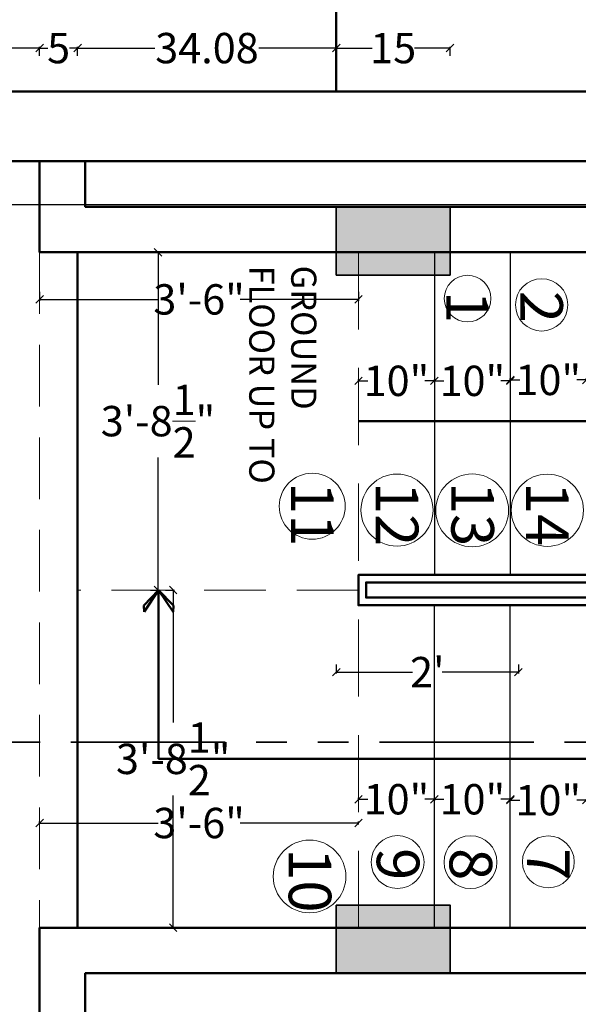
# Model space of a CAD drawing. Units: inches. Extents: x -60 to 284, y -245 to 257.
# Tile 7 of 10: x 25 to 99, y 12 to 141. Entities that reach past the tile are written whole.
import ezdxf

# ---------------------------------------------------------------- set-up
doc = ezdxf.new("R2010")
doc.units = ezdxf.units.IN
doc.header["$LTSCALE"] = 0.8
doc.header["$MEASUREMENT"] = 0
doc.linetypes.add('DASHED', pattern=[19.05, 12.7, -6.35])
doc.linetypes.add('PHANTOM', pattern=[63.5, 31.75, -6.35, 6.35, -6.35, 6.35, -6.35])
for name, color, linetype, lineweight in [('A-ANNO-DIMS', 2, 'Continuous', 18), ('A-ANNO-SECT', 1, 'PHANTOM', 35), ('A-ANNO-SYMB', 3, 'Continuous', 18), ('A-ANNO-TEXT', 3, 'Continuous', 18), ('A-ANNO-TTLB', 7, 'Continuous', 50), ('A-COLS', 1, 'Continuous', 35), ('A-FLOR-STRS', 4, 'Continuous', 25), ('A-FLOR-STRS-OVHD', 4, 'DASHED', 18), ('A-WALL', 7, 'Continuous', 50)]:
    doc.layers.add(name, color=color, linetype=linetype, lineweight=lineweight)
doc.styles.get("Standard").update_dxf_attribs({"font": 'arial.ttf'})
doc.dimstyles.get("Standard").update_dxf_attribs({"dimtxt": 4, "dimasz": 1, "dimexe": 0.18, "dimexo": 0.0625, "dimgap": 0.09, "dimtad": 0, "dimtih": 1, "dimtoh": 1, "dimzin": 0, "dimdsep": 46, "dimlunit": 4, "dimtxsty": 'Standard', "dimblk": 'OBLIQUE', "dimcen": 0.09, "dimadec": 0, "dimazin": 0, "dimtfac": 1, "dimtofl": 0, "dimtmove": 0, "dimatfit": 3, "dimfxl": 1, "dimfxlon": 1, "dimtolj": 1, "dimtzin": 0, "dimarcsym": 0})

# ---------------------------------------------------------------- blocks, each defined once
blk = doc.blocks.new('_Oblique')
at = {"color": 0, "linetype": 'ByBlock', "lineweight": -2}
blk.add_line((-0.5, -0.5), (0.5, 0.5), dxfattribs=at)
blk = doc.blocks.new('*D8')
at = {"layer": 'A-ANNO-DIMS', "color": 0, "lineweight": -2, "ltscale": 0.8, "transparency": 16777216}
for p, q in [((89.94, 38.48), (89.94, 38.66)), ((89.94, 38.48), (91.18, 38.48)), ((99.94, 38.48), (98.69, 38.48)), ((99.94, 38.6), (99.94, 38.3))]:
    blk.add_line(p, q, dxfattribs=at)
at = {"layer": 'Defpoints', "color": 0, "ltscale": 0.8, "transparency": 16777216}
for p in [(89.94, 38.48), (99.94, 38.66), (99.94, 38.48)]:
    blk.add_point(p, dxfattribs=at)
at = {"layer": 'A-ANNO-DIMS', "color": 0, "lineweight": -2, "ltscale": 0.8, "transparency": 16777216, "rotation": 180}
blk.add_blockref('_Oblique', (89.94, 38.48), dxfattribs=at)
at = {"layer": 'A-ANNO-DIMS', "color": 0, "lineweight": -2, "ltscale": 0.8, "transparency": 16777216}
blk.add_blockref('_Oblique', (99.94, 38.48), dxfattribs=at)
at = {"layer": 'A-ANNO-DIMS', "color": 0, "ltscale": 0.8, "transparency": 16777216, "insert": (94.94, 38.48), "char_height": 4, "attachment_point": 5}
blk.add_mtext('\\A1;10"', dxfattribs=at)
blk = doc.blocks.new('*D9')
at = {"layer": 'A-ANNO-DIMS', "color": 0, "lineweight": -2, "ltscale": 0.8, "transparency": 16777216}
for p, q in [((79.94, 38.54), (79.94, 38.78)), ((79.94, 38.6), (81.18, 38.6)), ((89.94, 38.6), (88.69, 38.6)), ((89.94, 38.6), (89.94, 38.78))]:
    blk.add_line(p, q, dxfattribs=at)
at = {"layer": 'Defpoints', "color": 0, "ltscale": 0.8, "transparency": 16777216}
for p in [(79.94, 38.48), (89.94, 38.6), (89.94, 38.6)]:
    blk.add_point(p, dxfattribs=at)
at = {"layer": 'A-ANNO-DIMS', "color": 0, "lineweight": -2, "ltscale": 0.8, "transparency": 16777216, "rotation": 180}
blk.add_blockref('_Oblique', (79.94, 38.6), dxfattribs=at)
at = {"layer": 'A-ANNO-DIMS', "color": 0, "lineweight": -2, "ltscale": 0.8, "transparency": 16777216}
blk.add_blockref('_Oblique', (89.94, 38.6), dxfattribs=at)
at = {"layer": 'A-ANNO-DIMS', "color": 0, "ltscale": 0.8, "transparency": 16777216, "insert": (84.94, 38.6), "char_height": 4, "attachment_point": 5}
blk.add_mtext('\\A1;10"', dxfattribs=at)
blk = doc.blocks.new('*D10')
at = {"layer": 'A-ANNO-DIMS', "color": 0, "lineweight": -2, "ltscale": 0.8, "transparency": 16777216}
for p, q in [((69.94, 38.6), (69.94, 38.78)), ((69.94, 38.6), (71.18, 38.6)), ((79.94, 38.6), (78.69, 38.6)), ((79.94, 38.72), (79.94, 38.42))]:
    blk.add_line(p, q, dxfattribs=at)
at = {"layer": 'Defpoints', "color": 0, "ltscale": 0.8, "transparency": 16777216}
for p in [(69.94, 38.6), (79.94, 38.78), (79.94, 38.6)]:
    blk.add_point(p, dxfattribs=at)
at = {"layer": 'A-ANNO-DIMS', "color": 0, "lineweight": -2, "ltscale": 0.8, "transparency": 16777216, "rotation": 180}
blk.add_blockref('_Oblique', (69.94, 38.6), dxfattribs=at)
at = {"layer": 'A-ANNO-DIMS', "color": 0, "lineweight": -2, "ltscale": 0.8, "transparency": 16777216}
blk.add_blockref('_Oblique', (79.94, 38.6), dxfattribs=at)
at = {"layer": 'A-ANNO-DIMS', "color": 0, "ltscale": 0.8, "transparency": 16777216, "insert": (74.94, 38.6), "char_height": 4, "attachment_point": 5}
blk.add_mtext('\\A1;10"', dxfattribs=at)
blk = doc.blocks.new('*D18')
at = {"layer": 'A-ANNO-DIMS', "color": 0, "lineweight": -2, "ltscale": 0.8, "transparency": 16777216}
for p, q in [((89.94, 93.85), (89.94, 94.03)), ((89.94, 93.85), (91.18, 93.85)), ((99.94, 93.85), (98.69, 93.85)), ((99.94, 93.73), (99.94, 94.03))]:
    blk.add_line(p, q, dxfattribs=at)
at = {"layer": 'Defpoints', "color": 0, "ltscale": 0.8, "transparency": 16777216}
for p in [(89.94, 93.85), (99.94, 93.85), (99.94, 93.67)]:
    blk.add_point(p, dxfattribs=at)
at = {"layer": 'A-ANNO-DIMS', "color": 0, "lineweight": -2, "ltscale": 0.8, "transparency": 16777216, "rotation": 180}
blk.add_blockref('_Oblique', (89.94, 93.85), dxfattribs=at)
at = {"layer": 'A-ANNO-DIMS', "color": 0, "lineweight": -2, "ltscale": 0.8, "transparency": 16777216}
blk.add_blockref('_Oblique', (99.94, 93.85), dxfattribs=at)
at = {"layer": 'A-ANNO-DIMS', "color": 0, "ltscale": 0.8, "transparency": 16777216, "insert": (94.94, 93.85), "char_height": 4, "attachment_point": 5}
blk.add_mtext('\\A1;10"', dxfattribs=at)
blk = doc.blocks.new('*D19')
at = {"layer": 'A-ANNO-DIMS', "color": 0, "lineweight": -2, "ltscale": 0.8, "transparency": 16777216}
for p, q in [((79.94, 93.79), (79.94, 93.55)), ((79.94, 93.73), (81.18, 93.73)), ((89.94, 93.73), (88.69, 93.73)), ((89.94, 93.73), (89.94, 93.91))]:
    blk.add_line(p, q, dxfattribs=at)
at = {"layer": 'Defpoints', "color": 0, "ltscale": 0.8, "transparency": 16777216}
for p in [(79.94, 93.85), (89.94, 93.73), (89.94, 93.73)]:
    blk.add_point(p, dxfattribs=at)
at = {"layer": 'A-ANNO-DIMS', "color": 0, "lineweight": -2, "ltscale": 0.8, "transparency": 16777216, "rotation": 180}
blk.add_blockref('_Oblique', (79.94, 93.73), dxfattribs=at)
at = {"layer": 'A-ANNO-DIMS', "color": 0, "lineweight": -2, "ltscale": 0.8, "transparency": 16777216}
blk.add_blockref('_Oblique', (89.94, 93.73), dxfattribs=at)
at = {"layer": 'A-ANNO-DIMS', "color": 0, "ltscale": 0.8, "transparency": 16777216, "insert": (84.94, 93.73), "char_height": 4, "attachment_point": 5}
blk.add_mtext('\\A1;10"', dxfattribs=at)
blk = doc.blocks.new('*D11')
at = {"layer": 'A-ANNO-DIMS', "color": 0, "lineweight": -2, "ltscale": 0.8, "transparency": 16777216}
for p, q in [((69.94, 93.73), (69.94, 93.91)), ((69.94, 93.73), (71.18, 93.73)), ((79.94, 93.73), (78.69, 93.73)), ((79.94, 93.61), (79.94, 93.91))]:
    blk.add_line(p, q, dxfattribs=at)
at = {"layer": 'Defpoints', "color": 0, "ltscale": 0.8, "transparency": 16777216}
for p in [(69.94, 93.73), (79.94, 93.73), (79.94, 93.55)]:
    blk.add_point(p, dxfattribs=at)
at = {"layer": 'A-ANNO-DIMS', "color": 0, "lineweight": -2, "ltscale": 0.8, "transparency": 16777216, "rotation": 180}
blk.add_blockref('_Oblique', (69.94, 93.73), dxfattribs=at)
at = {"layer": 'A-ANNO-DIMS', "color": 0, "lineweight": -2, "ltscale": 0.8, "transparency": 16777216}
blk.add_blockref('_Oblique', (79.94, 93.73), dxfattribs=at)
at = {"layer": 'A-ANNO-DIMS', "color": 0, "ltscale": 0.8, "transparency": 16777216, "insert": (74.94, 93.73), "char_height": 4, "attachment_point": 5}
blk.add_mtext('\\A1;10"', dxfattribs=at)
blk = doc.blocks.new('*D20')
at = {"layer": 'A-ANNO-DIMS', "color": 0, "lineweight": -2, "ltscale": 0.8, "transparency": 16777216}
for p, q in [((27.94, 105.46), (27.94, 104.28)), ((69.94, 105.46), (69.94, 104.28)), ((27.94, 104.46), (43.53, 104.46)), ((69.94, 104.46), (54.34, 104.46))]:
    blk.add_line(p, q, dxfattribs=at)
at = {"layer": 'Defpoints', "color": 0, "ltscale": 0.8, "transparency": 16777216}
for p in [(27.94, 107.07), (69.94, 107.07), (69.94, 104.46)]:
    blk.add_point(p, dxfattribs=at)
at = {"layer": 'A-ANNO-DIMS', "color": 0, "lineweight": -2, "ltscale": 0.8, "transparency": 16777216, "rotation": 180}
blk.add_blockref('_Oblique', (27.94, 104.46), dxfattribs=at)
at = {"layer": 'A-ANNO-DIMS', "color": 0, "lineweight": -2, "ltscale": 0.8, "transparency": 16777216}
blk.add_blockref('_Oblique', (69.94, 104.46), dxfattribs=at)
at = {"layer": 'A-ANNO-DIMS', "color": 0, "ltscale": 0.8, "transparency": 16777216, "insert": (48.94, 104.46), "char_height": 4, "attachment_point": 5}
blk.add_mtext('\\A1;3\'-6"', dxfattribs=at)
blk = doc.blocks.new('*D21')
at = {"layer": 'A-ANNO-DIMS', "color": 0, "lineweight": -2, "ltscale": 0.8, "transparency": 16777216}
for p, q in [((27.94, 35.29), (27.94, 35.65)), ((27.94, 35.47), (43.53, 35.47)), ((69.94, 35.47), (54.34, 35.47)), ((69.94, 35.29), (69.94, 35.65))]:
    blk.add_line(p, q, dxfattribs=at)
at = {"layer": 'Defpoints', "color": 0, "ltscale": 0.8, "transparency": 16777216}
for p in [(27.94, 35.23), (69.94, 35.47), (69.94, 35.23)]:
    blk.add_point(p, dxfattribs=at)
at = {"layer": 'A-ANNO-DIMS', "color": 0, "lineweight": -2, "ltscale": 0.8, "transparency": 16777216, "rotation": 180}
blk.add_blockref('_Oblique', (27.94, 35.47), dxfattribs=at)
at = {"layer": 'A-ANNO-DIMS', "color": 0, "lineweight": -2, "ltscale": 0.8, "transparency": 16777216}
blk.add_blockref('_Oblique', (69.94, 35.47), dxfattribs=at)
at = {"layer": 'A-ANNO-DIMS', "color": 0, "ltscale": 0.8, "transparency": 16777216, "insert": (48.94, 35.47), "char_height": 4, "attachment_point": 5}
blk.add_mtext('\\A1;3\'-6"', dxfattribs=at)
blk = doc.blocks.new('*D24')
at = {"layer": 'A-ANNO-DIMS', "color": 0, "lineweight": -2, "ltscale": 0.8, "transparency": 16777216}
for p, q in [((44.53, 66.17), (45.71, 66.17)), ((45.53, 66.17), (45.53, 48.72)), ((45.53, 21.67), (45.53, 39.11)), ((44.53, 21.67), (45.71, 21.67))]:
    blk.add_line(p, q, dxfattribs=at)
at = {"layer": 'Defpoints', "color": 0, "ltscale": 0.8, "transparency": 16777216}
for p in [(37.94, 66.17), (45.53, 66.17), (37.94, 21.67)]:
    blk.add_point(p, dxfattribs=at)
at = {"layer": 'A-ANNO-DIMS', "color": 0, "lineweight": -2, "ltscale": 0.8, "transparency": 16777216}
for p, rotation in [((45.53, 66.17), 90), ((45.53, 21.67), 270)]:
    blk.add_blockref('_Oblique', p, dxfattribs=dict(at, rotation=rotation))
at = {"layer": 'A-ANNO-DIMS', "color": 0, "ltscale": 0.8, "transparency": 16777216, "insert": (45.53, 43.92), "char_height": 4, "attachment_point": 5}
blk.add_mtext('\\A1;3\'-8{\\H1x;\\S1/2;}"', dxfattribs=at)
blk = doc.blocks.new('*D25')
at = {"layer": 'A-ANNO-DIMS', "color": 0, "lineweight": -2, "ltscale": 0.8, "transparency": 16777216}
for p, q in [((42.53, 110.67), (43.71, 110.67)), ((43.53, 110.67), (43.53, 93.22)), ((43.53, 66.17), (43.53, 83.61)), ((42.53, 66.17), (43.71, 66.17))]:
    blk.add_line(p, q, dxfattribs=at)
at = {"layer": 'Defpoints', "color": 0, "ltscale": 0.8, "transparency": 16777216}
for p in [(37.94, 110.67), (43.53, 110.67), (37.94, 66.17)]:
    blk.add_point(p, dxfattribs=at)
at = {"layer": 'A-ANNO-DIMS', "color": 0, "lineweight": -2, "ltscale": 0.8, "transparency": 16777216}
for p, rotation in [((43.53, 110.67), 90), ((43.53, 66.17), 270)]:
    blk.add_blockref('_Oblique', p, dxfattribs=dict(at, rotation=rotation))
at = {"layer": 'A-ANNO-DIMS', "color": 0, "ltscale": 0.8, "transparency": 16777216, "insert": (43.53, 88.42), "char_height": 4, "attachment_point": 5}
blk.add_mtext('\\A1;3\'-8{\\H1x;\\S1/2;}"', dxfattribs=at)
blk = doc.blocks.new('*D38')
at = {"layer": 'A-ANNO-DIMS', "color": 0, "lineweight": -2, "ltscale": 0.8, "transparency": 16777216}
for p, q in [((67.01, 56.35), (67.01, 55.17)), ((91.01, 56.35), (91.01, 55.17)), ((67.01, 55.35), (77.05, 55.35)), ((91.01, 55.35), (80.98, 55.35))]:
    blk.add_line(p, q, dxfattribs=at)
at = {"layer": 'Defpoints', "color": 0, "ltscale": 0.8, "transparency": 16777216}
for p in [(67.01, 57.45), (91.01, 57.45), (91.01, 55.35)]:
    blk.add_point(p, dxfattribs=at)
at = {"layer": 'A-ANNO-DIMS', "color": 0, "lineweight": -2, "ltscale": 0.8, "transparency": 16777216, "rotation": 180}
blk.add_blockref('_Oblique', (67.01, 55.35), dxfattribs=at)
at = {"layer": 'A-ANNO-DIMS', "color": 0, "lineweight": -2, "ltscale": 0.8, "transparency": 16777216}
blk.add_blockref('_Oblique', (91.01, 55.35), dxfattribs=at)
at = {"layer": 'A-ANNO-DIMS', "color": 0, "ltscale": 0.8, "transparency": 16777216, "insert": (79.01, 55.35), "char_height": 4, "attachment_point": 5}
blk.add_mtext("\\A1;2'", dxfattribs=at)
blk = doc.blocks.new('*D76')
at = {"layer": 'A-ANNO-DIMS', "color": 0, "lineweight": -2, "ltscale": 0.8, "transparency": 16777216}
for p, q in [((-0.88, 117.95), (-0.88, 116.77)), ((-0.88, 116.95), (107.9, 116.95)), ((230.43, 116.95), (121.65, 116.95)), ((230.43, 117.95), (230.43, 116.77))]:
    blk.add_line(p, q, dxfattribs=at)
at = {"layer": 'Defpoints', "color": 0, "ltscale": 0.8, "transparency": 16777216}
for p in [(-0.88, 131.85), (230.43, 131.85), (230.43, 116.95)]:
    blk.add_point(p, dxfattribs=at)
at = {"layer": 'A-ANNO-DIMS', "color": 0, "lineweight": -2, "ltscale": 0.8, "transparency": 16777216, "rotation": 180}
blk.add_blockref('_Oblique', (-0.88, 116.95), dxfattribs=at)
at = {"layer": 'A-ANNO-DIMS', "color": 0, "lineweight": -2, "ltscale": 0.8, "transparency": 16777216}
blk.add_blockref('_Oblique', (230.43, 116.95), dxfattribs=at)
at = {"layer": 'A-ANNO-DIMS', "color": 0, "ltscale": 0.8, "transparency": 16777216, "insert": (114.78, 116.95), "char_height": 4, "attachment_point": 5}
blk.add_mtext('\\A1;231.3', dxfattribs=at)
blk = doc.blocks.new('*D91')
at = {"layer": 'A-ANNO-DIMS', "color": 0, "lineweight": -2, "ltscale": 0.8, "transparency": 16777216}
for p, q in [((0.09, 136.57), (0.09, 137.75)), ((0.09, 137.57), (7.12, 137.57)), ((27.94, 137.57), (20.9, 137.57)), ((27.94, 136.57), (27.94, 137.75))]:
    blk.add_line(p, q, dxfattribs=at)
at = {"layer": 'Defpoints', "color": 0, "ltscale": 0.8, "transparency": 16777216}
for p in [(27.94, 137.57), (0.09, 122.67), (27.94, 122.67)]:
    blk.add_point(p, dxfattribs=at)
at = {"layer": 'A-ANNO-DIMS', "color": 0, "lineweight": -2, "ltscale": 0.8, "transparency": 16777216, "rotation": 180}
blk.add_blockref('_Oblique', (0.09, 137.57), dxfattribs=at)
at = {"layer": 'A-ANNO-DIMS', "color": 0, "lineweight": -2, "ltscale": 0.8, "transparency": 16777216}
blk.add_blockref('_Oblique', (27.94, 137.57), dxfattribs=at)
at = {"layer": 'A-ANNO-DIMS', "color": 0, "ltscale": 0.8, "transparency": 16777216, "insert": (14.01, 137.57), "char_height": 4, "attachment_point": 5}
blk.add_mtext('\\A1;27.85', dxfattribs=at)
blk = doc.blocks.new('*D92')
at = {"layer": 'A-ANNO-DIMS', "color": 0, "lineweight": -2, "ltscale": 0.8, "transparency": 16777216}
for p, q in [((27.94, 136.57), (27.94, 137.75)), ((27.94, 137.57), (29.02, 137.57)), ((32.94, 137.57), (31.85, 137.57)), ((32.94, 136.57), (32.94, 137.75))]:
    blk.add_line(p, q, dxfattribs=at)
at = {"layer": 'Defpoints', "color": 0, "ltscale": 0.8, "transparency": 16777216}
for p in [(32.94, 137.57), (27.94, 122.67), (32.94, 110.67)]:
    blk.add_point(p, dxfattribs=at)
at = {"layer": 'A-ANNO-DIMS', "color": 0, "lineweight": -2, "ltscale": 0.8, "transparency": 16777216, "rotation": 180}
blk.add_blockref('_Oblique', (27.94, 137.57), dxfattribs=at)
at = {"layer": 'A-ANNO-DIMS', "color": 0, "lineweight": -2, "ltscale": 0.8, "transparency": 16777216}
blk.add_blockref('_Oblique', (32.94, 137.57), dxfattribs=at)
at = {"layer": 'A-ANNO-DIMS', "color": 0, "ltscale": 0.8, "transparency": 16777216, "insert": (30.44, 137.57), "char_height": 4, "attachment_point": 5}
blk.add_mtext('\\A1;5', dxfattribs=at)
blk = doc.blocks.new('*D93')
at = {"layer": 'A-ANNO-DIMS', "color": 0, "lineweight": -2, "ltscale": 0.8, "transparency": 16777216}
for p, q in [((32.94, 136.57), (32.94, 137.75)), ((32.94, 137.57), (43.13, 137.57)), ((67.01, 137.57), (56.82, 137.57)), ((67.01, 136.57), (67.01, 137.75))]:
    blk.add_line(p, q, dxfattribs=at)
at = {"layer": 'Defpoints', "color": 0, "ltscale": 0.8, "transparency": 16777216}
for p in [(67.01, 137.57), (32.94, 110.67), (67.01, 107.67)]:
    blk.add_point(p, dxfattribs=at)
at = {"layer": 'A-ANNO-DIMS', "color": 0, "lineweight": -2, "ltscale": 0.8, "transparency": 16777216, "rotation": 180}
blk.add_blockref('_Oblique', (32.94, 137.57), dxfattribs=at)
at = {"layer": 'A-ANNO-DIMS', "color": 0, "lineweight": -2, "ltscale": 0.8, "transparency": 16777216}
blk.add_blockref('_Oblique', (67.01, 137.57), dxfattribs=at)
at = {"layer": 'A-ANNO-DIMS', "color": 0, "ltscale": 0.8, "transparency": 16777216, "insert": (49.98, 137.57), "char_height": 4, "attachment_point": 5}
blk.add_mtext('\\A1;34.08', dxfattribs=at)
blk = doc.blocks.new('*D94')
at = {"layer": 'A-ANNO-DIMS', "color": 0, "lineweight": -2, "ltscale": 0.8, "transparency": 16777216}
for p, q in [((67.01, 136.57), (67.01, 137.75)), ((67.01, 137.57), (71.73, 137.57)), ((82.01, 137.57), (77.3, 137.57)), ((82.01, 136.57), (82.01, 137.75))]:
    blk.add_line(p, q, dxfattribs=at)
at = {"layer": 'Defpoints', "color": 0, "ltscale": 0.8, "transparency": 16777216}
for p in [(82.01, 137.57), (67.01, 107.67), (82.01, 107.67)]:
    blk.add_point(p, dxfattribs=at)
at = {"layer": 'A-ANNO-DIMS', "color": 0, "lineweight": -2, "ltscale": 0.8, "transparency": 16777216, "rotation": 180}
blk.add_blockref('_Oblique', (67.01, 137.57), dxfattribs=at)
at = {"layer": 'A-ANNO-DIMS', "color": 0, "lineweight": -2, "ltscale": 0.8, "transparency": 16777216}
blk.add_blockref('_Oblique', (82.01, 137.57), dxfattribs=at)
at = {"layer": 'A-ANNO-DIMS', "color": 0, "ltscale": 0.8, "transparency": 16777216, "insert": (74.51, 137.57), "char_height": 4, "attachment_point": 5}
blk.add_mtext('\\A1;15', dxfattribs=at)
blk = doc.blocks.new('*D99')
at = {"layer": 'A-ANNO-DIMS', "color": 0, "lineweight": -2, "ltscale": 0.8, "transparency": 16777216}
for p, q in [((-42.73, 122.67), (-43.91, 122.67)), ((-43.73, 122.67), (-43.73, 121.8)), ((-43.73, 116.67), (-43.73, 117.53)), ((-42.73, 116.67), (-43.91, 116.67))]:
    blk.add_line(p, q, dxfattribs=at)
at = {"layer": 'Defpoints', "color": 0, "ltscale": 0.8, "transparency": 16777216}
for p in [(-43.73, 122.67), (33.94, 122.67), (33.94, 116.67)]:
    blk.add_point(p, dxfattribs=at)
at = {"layer": 'A-ANNO-DIMS', "color": 0, "lineweight": -2, "ltscale": 0.8, "transparency": 16777216}
for p, rotation in [((-43.73, 122.67), 90), ((-43.73, 116.67), 270)]:
    blk.add_blockref('_Oblique', p, dxfattribs=dict(at, rotation=rotation))
at = {"layer": 'A-ANNO-DIMS', "color": 0, "ltscale": 0.8, "transparency": 16777216, "insert": (-43.73, 119.67), "char_height": 4, "attachment_point": 5}
blk.add_mtext('\\A1;6', dxfattribs=at)
blk = doc.blocks.new('*D100')
at = {"layer": 'A-ANNO-DIMS', "color": 0, "lineweight": -2, "ltscale": 0.8, "transparency": 16777216}
for p, q in [((-42.73, 116.67), (-43.91, 116.67)), ((-43.73, 116.67), (-43.73, 115.8)), ((-42.73, 110.67), (-43.91, 110.67)), ((-43.73, 110.67), (-43.73, 111.53))]:
    blk.add_line(p, q, dxfattribs=at)
at = {"layer": 'Defpoints', "color": 0, "ltscale": 0.8, "transparency": 16777216}
for p in [(-43.73, 116.67), (33.94, 116.67), (32.94, 110.67)]:
    blk.add_point(p, dxfattribs=at)
at = {"layer": 'A-ANNO-DIMS', "color": 0, "lineweight": -2, "ltscale": 0.8, "transparency": 16777216}
for p, rotation in [((-43.73, 116.67), 90), ((-43.73, 110.67), 270)]:
    blk.add_blockref('_Oblique', p, dxfattribs=dict(at, rotation=rotation))
at = {"layer": 'A-ANNO-DIMS', "color": 0, "ltscale": 0.8, "transparency": 16777216, "insert": (-43.73, 113.67), "char_height": 4, "attachment_point": 5}
blk.add_mtext('\\A1;6', dxfattribs=at)
blk = doc.blocks.new('*D101')
at = {"layer": 'A-ANNO-DIMS', "color": 0, "lineweight": -2, "ltscale": 0.8, "transparency": 16777216}
for p, q in [((-42.73, 15.67), (-43.91, 15.67)), ((-43.73, 15.67), (-43.73, 14.8)), ((-43.73, 9.67), (-43.73, 10.53)), ((-42.73, 9.67), (-43.91, 9.67))]:
    blk.add_line(p, q, dxfattribs=at)
at = {"layer": 'Defpoints', "color": 0, "ltscale": 0.8, "transparency": 16777216}
for p in [(-43.73, 15.67), (33.94, 15.67), (33.94, 9.67)]:
    blk.add_point(p, dxfattribs=at)
at = {"layer": 'A-ANNO-DIMS', "color": 0, "lineweight": -2, "ltscale": 0.8, "transparency": 16777216}
for p, rotation in [((-43.73, 15.67), 90), ((-43.73, 9.67), 270)]:
    blk.add_blockref('_Oblique', p, dxfattribs=dict(at, rotation=rotation))
at = {"layer": 'A-ANNO-DIMS', "color": 0, "ltscale": 0.8, "transparency": 16777216, "insert": (-43.73, 12.67), "char_height": 4, "attachment_point": 5}
blk.add_mtext('\\A1;6', dxfattribs=at)
blk = doc.blocks.new('*D102')
at = {"layer": 'A-ANNO-DIMS', "color": 0, "lineweight": -2, "ltscale": 0.8, "transparency": 16777216}
for p, q in [((-42.73, 21.67), (-43.91, 21.67)), ((-43.73, 21.67), (-43.73, 20.8)), ((-42.73, 15.67), (-43.91, 15.67)), ((-43.73, 15.67), (-43.73, 16.53))]:
    blk.add_line(p, q, dxfattribs=at)
at = {"layer": 'Defpoints', "color": 0, "ltscale": 0.8, "transparency": 16777216}
for p in [(32.94, 21.67), (-43.73, 15.67), (33.94, 15.67)]:
    blk.add_point(p, dxfattribs=at)
at = {"layer": 'A-ANNO-DIMS', "color": 0, "lineweight": -2, "ltscale": 0.8, "transparency": 16777216}
for p, rotation in [((-43.73, 21.67), 90), ((-43.73, 15.67), 270)]:
    blk.add_blockref('_Oblique', p, dxfattribs=dict(at, rotation=rotation))
at = {"layer": 'A-ANNO-DIMS', "color": 0, "ltscale": 0.8, "transparency": 16777216, "insert": (-43.73, 18.67), "char_height": 4, "attachment_point": 5}
blk.add_mtext('\\A1;6', dxfattribs=at)

msp = doc.modelspace()

# ---------------------------------------------------------------- hatches: boundary and pattern name
at = {"layer": 'A-COLS', "ltscale": 0.8}
h = msp.add_hatch(color=256, dxfattribs=at)
h.dxf.hatch_style = 1
h.paths.add_polyline_path([(82.0139, 116.666), (67.0139, 116.666), (67.0139, 107.666), (82.0139, 107.666)])
h = msp.add_hatch(color=256, dxfattribs=at)
h.dxf.hatch_style = 1
h.paths.add_polyline_path([(82.0139, 24.666), (67.0139, 24.666), (67.0139, 15.666), (82.0139, 15.666)])

# ---------------------------------------------------------------- linework, layer by layer
at = {"layer": 'A-ANNO-SECT', "ltscale": 0.8}
msp.add_line((255.5807, 46.116), (-23.5489, 46.116), dxfattribs=at)
at = {"layer": 'A-ANNO-SYMB', "ltscale": 0.8}
for centre, radius in [((84.3072, 104.5638), 3.069), ((94.0706, 103.74), 3.4482), ((63.8472, 77.2069), 4.347), ((75.0147, 76.6947), 4.7439), ((84.9195, 76.666), 4.7968), ((94.8158, 76.6775), 4.7576), ((75.094, 30.3238), 3.4808), ((84.6889, 30.32), 3.4829), ((94.9441, 30.3524), 3.4155), ((63.4942, 28.4258), 4.788)]:
    msp.add_circle(centre, radius, dxfattribs=at)
at = {"layer": 'A-ANNO-TTLB', "ltscale": 0.8}
for points in [[(-0.8787, 239.5184), (230.4297, 239.5184), (230.4297, 131.8542), (-0.8787, 131.8542)], [(0.0867, 122.666), (239.6639, 122.666), (239.6639, 9.666), (0.0867, 9.666)]]:
    msp.add_lwpolyline(points, close=True, dxfattribs=at)
at = {"layer": 'A-COLS', "ltscale": 0.8}
for points in [[(67.0139, 116.666), (82.0139, 116.666), (82.0139, 107.666), (67.0139, 107.666)], [(67.0139, 24.666), (82.0139, 24.666), (82.0139, 15.666), (67.0139, 15.666)]]:
    msp.add_lwpolyline(points, close=True, dxfattribs=at)
at = {"layer": 'A-FLOR-STRS'}
for p, q in [((79.9361, 110.666), (79.9361, 68.166)), ((89.9361, 110.666), (89.9361, 68.166)), ((79.9361, 21.666), (79.9361, 64.166)), ((89.9361, 21.666), (89.9361, 64.166))]:
    msp.add_line(p, q, dxfattribs=at)
at = {"layer": 'A-FLOR-STRS-OVHD', "ltscale": 0.8}
for p, q in [((27.9361, 110.666), (27.9361, 21.666)), ((69.9361, 66.166), (32.9361, 66.166))]:
    msp.add_line(p, q, dxfattribs=at)
at = {"layer": 'A-FLOR-STRS-OVHD'}
for p in [(69.9361, 110.666), (69.9361, 21.666)]:
    msp.add_line(p, (69.9361, 66.166), dxfattribs=at)
at = {"layer": 'A-WALL', "ltscale": 0.8}
for p, q in [((67.0139, 131.8542), (67.0139, 239.5184)), ((32.9361, 110.666), (32.9361, 21.666)), ((69.9361, 88.416), (159.9361, 88.416)), ((41.6712, 64.1216), (43.6123, 66.166)), ((43.6123, 66.166), (41.6983, 63.2855)), ((43.6123, 43.916), (43.6123, 66.166)), ((43.6123, 66.166), (45.5263, 63.2855)), ((45.5535, 64.1216), (43.6123, 66.166)), ((41.6983, 63.2855), (41.6712, 64.1216)), ((45.5263, 63.2855), (45.5535, 64.1216)), ((168.271, 43.916), (43.6123, 43.916))]:
    msp.add_line(p, q, dxfattribs=at)
at = {"layer": 'A-WALL'}
for points in [[(198.9361, 116.666), (198.9361, 110.666), (159.9361, 110.666), (79.9361, 110.666), (37.9361, 110.666), (27.9361, 110.666), (27.9361, 122.666)], [(192.9361, 116.666), (159.9361, 116.666), (79.9361, 116.666), (37.9361, 116.666), (33.9361, 116.666), (33.9361, 122.666)], [(198.9361, 9.666), (198.9361, 21.666), (159.9361, 21.666), (79.9361, 21.666), (37.9361, 21.666), (27.9361, 21.666), (27.9361, 9.666)], [(192.9361, 9.666), (192.9361, 15.666), (159.9361, 15.666), (79.9361, 15.666), (37.9361, 15.666), (33.9361, 15.666), (33.9361, 9.666)]]:
    msp.add_lwpolyline(points, dxfattribs=at)
for points in [[(159.9361, 68.166), (69.9361, 68.166), (69.9361, 64.166), (159.9361, 64.166)], [(158.9361, 67.166), (70.9361, 67.166), (70.9361, 65.166), (158.9361, 65.166)]]:
    msp.add_lwpolyline(points, close=True, dxfattribs=at)

# ---------------------------------------------------------------- texts
at = {"layer": 'A-ANNO-TEXT', "ltscale": 0.8, "rotation": 270}
for s, width, gutter_width, insert, char_height, attachment_point in [('\\A1;GROUND \\PFLOOR UP TO', 69.138891, 0.3685, (64.3973, 108.9153), 3.316205, 1), ('2', 28.020867, 2.8021, (91.2571, 105.596), 5.6042, 7), ('1', 28.020867, 2.8021, (81.4936, 105.596), 5.6042, 7), ('11', 28.020867, 2.8021, (66.6607, 80.4161), 5.60417, 1), ('12', 28.020867, 2.8021, (77.8283, 80.4161), 5.60417, 1), ('13', 28.020867, 2.8021, (87.7828, 80.4161), 5.60417, 1), ('14', 28.020867, 2.8021, (97.6293, 80.4161), 5.60417, 1), ('10', 28.020867, 2.8021, (66.3555, 32.1663), 5.60417, 1), ('9', 28.020867, 2.8021, (77.9553, 32.1663), 5.6042, 1), ('8', 28.020867, 2.8021, (87.5502, 32.1663), 5.6042, 1), ('7', 28.020867, 2.8021, (97.7462, 32.1663), 5.6042, 1)]:
    msp.add_mtext_dynamic_manual_height_columns(s, width=width, gutter_width=gutter_width, heights=[0], dxfattribs=dict(at, insert=insert, char_height=char_height, attachment_point=attachment_point))

# ---------------------------------------------------------------- dimensions: what is measured, and where the dimension line sits
at = {"layer": 'A-ANNO-DIMS', "ltscale": 0.8}
for base, p1, p2, override, picture, middle in [((27.9361, 137.566), (0.0867, 122.666), (27.9361, 122.666), {"dimdec": 2, "dimlfac": 1, "dimrnd": 0, "dimzin": 0, "dimdsep": 46, "dimlunit": 2}, '*D91', (14.0114, 137.566)), ((32.9361, 137.566), (27.9361, 122.666), (32.9361, 110.666), {"dimdec": 0, "dimlfac": 1, "dimrnd": 0, "dimzin": 0, "dimdsep": 46, "dimlunit": 2}, '*D92', (30.4361, 137.566)), ((67.0139, 137.566), (32.9361, 110.666), (67.0139, 107.666), {"dimdec": 2, "dimlfac": 1, "dimrnd": 0, "dimzin": 0, "dimdsep": 46, "dimlunit": 2}, '*D93', (49.975, 137.566)), ((82.0139, 137.566), (67.0139, 107.666), (82.0139, 107.666), {"dimdec": 0, "dimlfac": 1, "dimrnd": 0, "dimzin": 0, "dimdsep": 46, "dimlunit": 2}, '*D94', (74.5139, 137.566)), ((230.4297, 116.9542), (-0.8787, 131.8542), (230.4297, 131.8542), {"dimdec": 1, "dimlfac": 1, "dimrnd": 0, "dimzin": 0, "dimdsep": 46, "dimlunit": 2}, '*D76', (114.7755, 116.9542)), ((69.9361, 104.4592), (27.9361, 107.0658), (69.9361, 107.0658), {"dimclrd": 0, "dimclre": 0, "dimclrt": 0}, '*D20', (48.9361, 104.4592)), ((79.9361, 93.7305), (69.9361, 93.7305), (79.9361, 93.5505), {"dimclrd": 0, "dimclre": 0, "dimclrt": 0}, '*D11', (74.9361, 93.7305)), ((89.9361, 93.7305), (79.9361, 93.8517), (89.9361, 93.7305), {"dimclrd": 0, "dimclre": 0, "dimclrt": 0}, '*D19', (84.9361, 93.7305)), ((99.9361, 93.8517), (89.9361, 93.8517), (99.9361, 93.6717), {"dimclrd": 0, "dimclre": 0, "dimclrt": 0}, '*D18', (94.9361, 93.8517)), ((91.0139, 55.3468), (67.0139, 57.4508), (91.0139, 57.4508), {"dimclrd": 0, "dimclre": 0, "dimclrt": 0}, '*D38', (79.0139, 55.3468)), ((79.9361, 38.6016), (69.9361, 38.6016), (79.9361, 38.7816), {"dimclrd": 0, "dimclre": 0, "dimclrt": 0}, '*D10', (74.9361, 38.6016)), ((89.9361, 38.6016), (79.9361, 38.4804), (89.9361, 38.6016), {"dimclrd": 0, "dimclre": 0, "dimclrt": 0}, '*D9', (84.9361, 38.6016)), ((99.9361, 38.4804), (89.9361, 38.4804), (99.9361, 38.6604), {"dimclrd": 0, "dimclre": 0, "dimclrt": 0}, '*D8', (94.9361, 38.4804)), ((69.9361, 35.4658), (27.9361, 35.2297), (69.9361, 35.2297), {"dimclrd": 0, "dimclre": 0, "dimclrt": 0}, '*D21', (48.9361, 35.4658))]:
    dim = msp.add_linear_dim(base=base, p1=p1, p2=p2, dimstyle='Standard', override=override, dxfattribs=at)
    dim.commit()
    dim.dimension.update_dxf_attribs({"geometry": picture, "text_midpoint": middle})
for base, p1, p2, override, picture, middle in [((-43.7318, 122.666), (33.9361, 116.666), (33.9361, 122.666), {"dimdec": 0, "dimlfac": 1, "dimrnd": 0, "dimzin": 0, "dimdsep": 46, "dimlunit": 2}, '*D99', (-43.7318, 119.666)), ((-43.7318, 116.666), (32.9361, 110.666), (33.9361, 116.666), {"dimdec": 0, "dimlfac": 1, "dimrnd": 0, "dimzin": 0, "dimdsep": 46, "dimlunit": 2}, '*D100', (-43.7318, 113.666)), ((43.531, 110.666), (37.9361, 66.166), (37.9361, 110.666), {"dimclrd": 0, "dimclre": 0, "dimclrt": 0}, '*D25', (43.531, 88.416)), ((45.5263, 66.166), (37.9361, 21.666), (37.9361, 66.166), {"dimclrd": 0, "dimclre": 0, "dimclrt": 0}, '*D24', (45.5263, 43.916)), ((-43.7318, 15.666), (32.9361, 21.666), (33.9361, 15.666), {"dimdec": 0, "dimlfac": 1, "dimrnd": 0, "dimzin": 0, "dimdsep": 46, "dimlunit": 2}, '*D102', (-43.7318, 18.666)), ((-43.7318, 15.666), (33.9361, 9.666), (33.9361, 15.666), {"dimdec": 0, "dimlfac": 1, "dimrnd": 0, "dimzin": 0, "dimdsep": 46, "dimlunit": 2}, '*D101', (-43.7318, 12.666))]:
    dim = msp.add_linear_dim(base=base, p1=p1, p2=p2, angle=90, dimstyle='Standard', override=override, dxfattribs=at)
    dim.commit()
    dim.dimension.update_dxf_attribs({"geometry": picture, "text_midpoint": middle})

doc.saveas('drawing.dxf')
